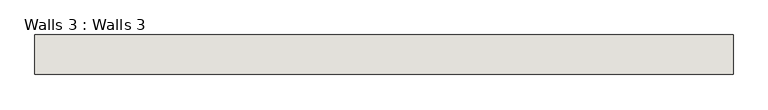
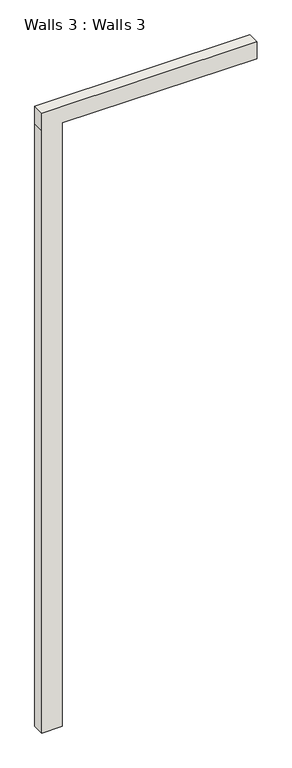
"""IFC4 building model written with IfcOpenShell, lengths in millimetres: wall geometry, Walls 3 : Walls 3."""

from ifc_helpers import new_model, si_unit, frame, origin, place, context, project, spatial, polyline, outline, extrude, source, transform, mapped, element, save


def walls_3_walls_3_bbde4dad(model_context):
    return source(origin(), model_context, "Body", "SweptSolid", [
        extrude(outline(polyline([(16422.5278597, -4957.5371298), (16422.5278597, -10348.6871298), (15956.2601563, -10348.6871298), (0.0, -10348.6871298), (0.0, -9834.3371298), (15981.6601563, -9834.3371298), (15981.6601563, -4957.5371298), (16422.5278597, -4957.5371298)])), frame((0.0, 636.5359817, 0.0), z_axis=(0.0, 1.0, 0.0), x_axis=(0.0, 0.0, 1.0)), (0.0, 0.0, 1.0), 304.8),
    ])


if __name__ == "__main__":
    model = new_model("IFC4")
    model_context = context("Model", 3, world=origin())
    ifc_project = project(units=[si_unit("LENGTHUNIT", "METRE", prefix="MILLI")], contexts=[model_context])
    site = spatial("IfcSite", under=ifc_project)
    building = spatial("IfcBuilding", under=site)
    placement = place(None, origin())
    walls_3_walls_3_shape = walls_3_walls_3_bbde4dad(model_context)
    element("IfcWall", 1, ObjectType="Walls 3 : Walls 3", at=placement, inside=building, context=model_context, shape_type="MappedRepresentation", body=[
        mapped(walls_3_walls_3_shape, transform((0.0, 0.0, 0.0), x_axis=(1.0, 0.0, 0.0), y_axis=(0.0, 1.0, 0.0), z_axis=(0.0, 0.0, 1.0))),
    ])
    save(model, "model.ifc")

# Revit data of these elements
# Element 1 (IfcWall, "Walls 3 : Walls 3")
#   Materials on its faces: "Default Wall"
# Materials
#   "Default Wall": colour RGB 128 128 128, transparency 0
